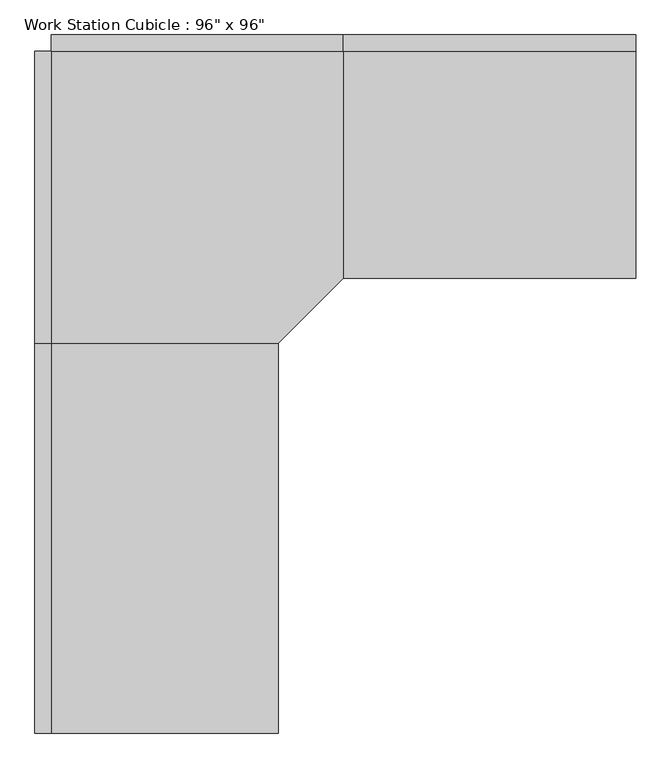
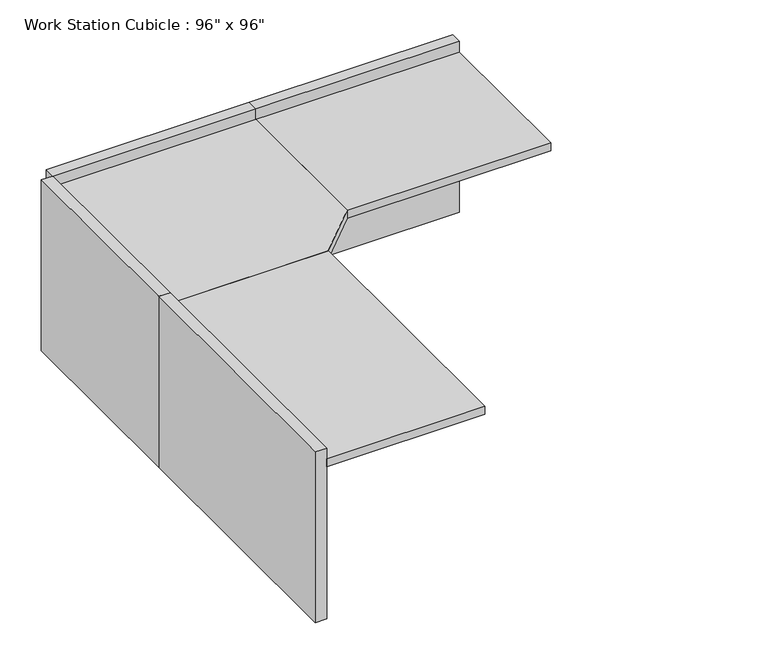
"""IFC4 building model written with IfcOpenShell, lengths in millimetres: furniture geometry."""

from ifc_helpers import new_model, si_unit, frame, origin, origin_with_axes, place, context, project, spatial, polyline, outline, extrude, source, transform, mapped, element, save


def furniture_5f8511dd(model_context):
    return source(origin(), model_context, "Body", "SweptSolid", [
        extrude(outline(polyline([(-80.9317522, -545.8230076), (833.4682478, -545.8230076), (833.4682478, -1257.0230076), (630.2682478, -1460.2230076), (-80.9317522, -1460.2230076), (-80.9317522, -545.8230076)])), frame((0.0, 0.0, 723.9), z_axis=(0.0, 0.0, 1.0), x_axis=(1.0, 0.0, 0.0)), (0.0, 0.0, 1.0), 38.1),
        extrude(outline(polyline([(630.2682478, -2679.4230076), (-80.9317522, -2679.4230076), (-80.9317522, -1460.2230076), (630.2682478, -1460.2230076), (630.2682478, -2679.4230076)])), frame((0.0, 0.0, 723.9), z_axis=(0.0, 0.0, 1.0), x_axis=(1.0, 0.0, 0.0)), (0.0, 0.0, 1.0), 38.1),
        extrude(outline(polyline([(1747.8682478, -1257.0230076), (833.4682478, -1257.0230076), (833.4682478, -545.8230076), (1747.8682478, -545.8230076), (1747.8682478, -1257.0230076)])), frame((0.0, 0.0, 723.9), z_axis=(0.0, 0.0, 1.0), x_axis=(1.0, 0.0, 0.0)), (0.0, 0.0, 1.0), 38.1),
        extrude(outline(polyline([(1747.8682478, -545.8230076), (833.4682478, -545.8230076), (833.4682478, -495.0230076), (1747.8682478, -495.0230076), (1747.8682478, -545.8230076)])), origin_with_axes(), (0.0, 0.0, 1.0), 812.8),
        extrude(outline(polyline([(833.4682478, -545.8230076), (-80.9317522, -545.8230076), (-80.9317522, -495.0230076), (833.4682478, -495.0230076), (833.4682478, -545.8230076)])), origin_with_axes(), (0.0, 0.0, 1.0), 812.8),
        extrude(outline(polyline([(-80.9317522, -1460.2230076), (-131.7317522, -1460.2230076), (-131.7317522, -545.8230076), (-80.9317522, -545.8230076), (-80.9317522, -1460.2230076)])), origin_with_axes(), (0.0, 0.0, 1.0), 812.8),
        extrude(outline(polyline([(-80.9317522, -2679.4230076), (-131.7317522, -2679.4230076), (-131.7317522, -1460.2230076), (-80.9317522, -1460.2230076), (-80.9317522, -2679.4230076)])), origin_with_axes(), (0.0, 0.0, 1.0), 812.8),
    ])


if __name__ == "__main__":
    model = new_model("IFC4")
    model_context = context("Model", 3, world=origin())
    ifc_project = project(units=[si_unit("LENGTHUNIT", "METRE", prefix="MILLI")], contexts=[model_context])
    site = spatial("IfcSite", under=ifc_project)
    building = spatial("IfcBuilding", under=site)
    placement = place(None, origin())
    furniture_shape = furniture_5f8511dd(model_context)
    element("IfcFurniture", 1, ObjectType="Work Station Cubicle : 96\" x 96\"", at=placement, inside=building, context=model_context, shape_type="MappedRepresentation", body=[
        mapped(furniture_shape, transform((0.0, 0.0, 0.0), x_axis=(1.0, 0.0, 0.0), y_axis=(0.0, 1.0, 0.0), z_axis=(0.0, 0.0, 1.0))),
    ])
    save(model, "model.ifc")

# Revit data of these elements
# Type "Work Station Cubicle : 96\" x 96\""
#   Assembly Code = "E2020"
#   Desktop Height = 2' - 6"
#   Desktop1 Width = 2' - 4"
#   Desktop2 Width = 2' - 4"
#   Panel Height = 2' - 8"
#   Panel1 Length = 4' - 0"
#   Panel2 Length = 3' - 0"
#   Cube Panel Material = Textile - Light Gray
#   Work Top Material = Laminate, Ivory, Matte
#   Default Elevation = 0
# Element 1 (IfcFurniture, "Work Station Cubicle : 96\" x 96\"")
#   Materials on its faces: "Textile - Light Gray", "Laminate, Ivory, Matte"
# Materials
#   "Textile - Light Gray": class "Fabric", colour RGB 204 204 204, transparency 0
#   "Laminate, Ivory, Matte": class "Plastic", colour RGB 247 247 239, transparency 0, Description = "Plastic Laminate - Ivory, Matte", Cost = 0
